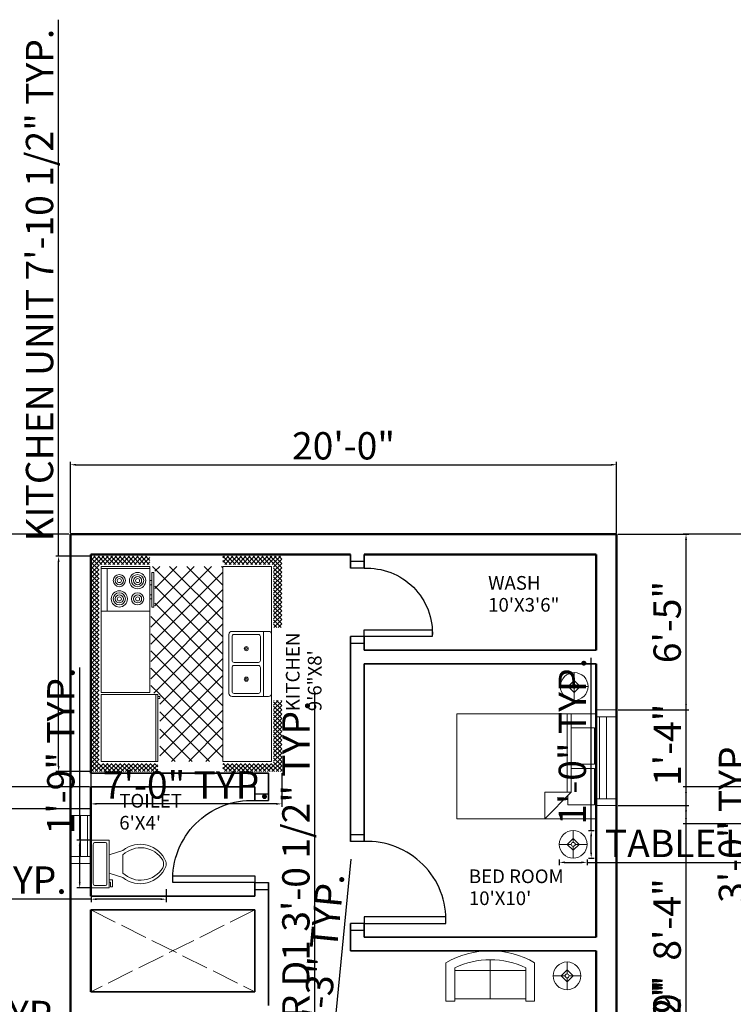
# Model space of a CAD drawing. Units: inches. Extents: x 2296 to 3335, y 495 to 1294.
# Tile 4 of 7: x 2638 to 2952, y 862 to 1294. Entities that reach past the tile are written whole.
import ezdxf

# ---------------------------------------------------------------- set-up
doc = ezdxf.new("R2010")
doc.units = ezdxf.units.IN
doc.linetypes.add('ACAD_ISO02W100', pattern=[15, 12, -3])
for name, color, linetype, lineweight in [('A-ANNO-DIMS', 2, 'Continuous', 18), ('A-AREA-IDEN', 7, 'Continuous', 18), ('A-FLOR-FIXT', 8, 'Continuous', 18), ('A-FLOR-OPEN', 7, 'ACAD_ISO02W100', 18), ('DOORS', 1, 'Continuous', 25), ('E-LITE', 2, 'Continuous', 18), ('FURNITURE', 2, 'Continuous', 18), ('INNER WALL', 6, 'Continuous', 35), ('OUTER WALL', 5, 'Continuous', 50), ('P-FIXT', 4, 'Continuous', 18), ('VENTILATOR', 4, 'Continuous', 18), ('WINDOWS', 3, 'Continuous', 18)]:
    doc.layers.add(name, color=color, linetype=linetype, lineweight=lineweight)
doc.styles.get("Standard").update_dxf_attribs({"font": 'arial.ttf'})
doc.dimstyles.new('ISO-25', dxfattribs={"dimtxt": 12, "dimasz": 2.5, "dimexe": 1.25, "dimexo": 0.625, "dimtad": 1, "dimdec": 1, "dimlunit": 3, "dimtxsty": 'Standard', "dimcen": 2.5, "dimadec": 0, "dimazin": 0, "dimtfac": 1, "dimtdec": 1, "dimtmove": 0, "dimatfit": 3, "dimfxl": 1, "dimarcsym": 0})

# ---------------------------------------------------------------- blocks, each defined once
blk = doc.blocks.new('Kitchen Layout - 7 x 8 ft')
for p, q in [((-5, 81.32), (2.68, 89)), ((-5, 83.44), (0.56, 89)), ((-5, 85.56), (-1.56, 89)), ((-5, 87.68), (-3.68, 89)), ((-1, 84.97), (-5, 88.97)), ((1.09, 85), (-2.91, 89)), ((3.21, 85), (-0.79, 89)), ((0.81, 85), (4.81, 89)), ((5.34, 85), (1.34, 89)), ((2.93, 85), (6.93, 89)), ((7.46, 85), (3.46, 89)), ((5.05, 85), (9.05, 89)), ((9.58, 85), (5.58, 89)), ((7.17, 85), (11.17, 89)), ((11.7, 85), (7.7, 89)), ((9.29, 85), (13.29, 89)), ((13.82, 85), (9.82, 89)), ((11.41, 85), (15.41, 89)), ((15.94, 85), (11.94, 89)), ((13.53, 85), (17.53, 89)), ((18.06, 85), (14.06, 89)), ((15.65, 85), (19.65, 89)), ((20.18, 85), (16.18, 89)), ((17.78, 85), (21.78, 89)), ((22.31, 85), (18.31, 89)), ((19.9, 85), (23.9, 89)), ((24.43, 85), (20.43, 89)), ((22.02, 85), (26.02, 89)), ((26.55, 85), (22.55, 89)), ((24.14, 85), (28.14, 89)), ((28.67, 85), (24.67, 89)), ((26.26, 85), (30.26, 89)), ((30.79, 85), (26.79, 89)), ((28.38, 85), (32.38, 89)), ((32.91, 85), (28.91, 89)), ((30.5, 85), (34.5, 89)), ((35.03, 85), (31.03, 89)), ((32.63, 85), (36.63, 89)), ((37.16, 85), (33.16, 89)), ((34.75, 85), (38.75, 89)), ((39.28, 85), (35.28, 89)), ((36.87, 85), (40.87, 89)), ((41.4, 85), (37.4, 89)), ((38.99, 85), (42.99, 89)), ((43.52, 85), (39.52, 89)), ((41.11, 85), (45.11, 89)), ((45.64, 85), (41.64, 89)), ((43.23, 85), (47.23, 89)), ((47.76, 85), (43.76, 89)), ((45.35, 85), (49.35, 89)), ((49.88, 85), (45.88, 89)), ((47.47, 85), (51.47, 89)), ((52, 85), (48, 89)), ((49.6, 85), (53.6, 89)), ((54.13, 85), (50.13, 89)), ((51.72, 85), (55.72, 89)), ((56.25, 85), (52.25, 89)), ((53.84, 85), (57.84, 89)), ((58.37, 85), (54.37, 89)), ((55.96, 85), (59.96, 89)), ((60.49, 85), (56.49, 89)), ((58.08, 85), (62.08, 89)), ((62.61, 85), (58.61, 89)), ((60.2, 85), (64.2, 89)), ((64.73, 85), (60.73, 89)), ((62.32, 85), (66.32, 89)), ((66.85, 85), (62.85, 89)), ((64.45, 85), (68.45, 89)), ((68.97, 85), (64.97, 89)), ((66.57, 85), (70.57, 89)), ((71.1, 85), (67.1, 89)), ((68.69, 85), (72.69, 89)), ((73.22, 85), (69.22, 89)), ((70.81, 85), (74.81, 89)), ((75.34, 85), (71.34, 89)), ((72.93, 85), (76.93, 89)), ((77.46, 85), (73.46, 89)), ((75.05, 85), (79.05, 89)), ((79.58, 85), (75.58, 89)), ((77.17, 85), (81.17, 89)), ((81.7, 85), (77.7, 89)), ((79.29, 85), (83.29, 89)), ((83.82, 85), (79.82, 89)), ((81.42, 85), (85.42, 89)), ((85.95, 85), (81.95, 89)), ((83.54, 85), (87.54, 89)), ((88.07, 85), (84.07, 89)), ((85.66, 85), (89.66, 89)), ((90.19, 85), (86.19, 89)), ((87.78, 85), (91.78, 89)), ((92.31, 85), (88.31, 89)), ((89.9, 85), (93.9, 89)), ((94.43, 85), (90.43, 89)), ((92.02, 85), (96.02, 89)), ((96.55, 85), (92.55, 89)), ((94.14, 85), (98.14, 89)), ((101, 82.67), (94.67, 89)), ((96.27, 85), (100.27, 89)), ((101, 84.79), (96.79, 89)), ((97, 83.61), (101, 87.61)), ((101, 86.92), (98.92, 89)), ((-1, 82.85), (-5, 86.85)), ((-1, 80.73), (-5, 84.73)), ((-5, 79.19), (-1, 83.19)), ((-1, 78.61), (-5, 82.61)), ((34, 84), (96, 84)), ((34, 60), (34, 84)), ((96, 84), (96, 60)), ((97, 81.49), (101, 85.49)), ((101, 80.55), (97, 84.55)), ((97, 79.37), (101, 83.37)), ((101, 78.43), (97, 82.43)), ((-5, 77.07), (-1, 81.07)), ((-1, 76.49), (-5, 80.49)), ((-5, 74.95), (-1, 78.95)), ((-1, 74.36), (-5, 78.36)), ((74, 81), (95, 81)), ((97, 77.25), (101, 81.25)), ((101, 76.31), (97, 80.31)), ((97, 75.13), (101, 79.13)), ((101, 74.19), (97, 78.19)), ((-5, 72.83), (-1, 76.83)), ((-1, 72.24), (-5, 76.24)), ((-5, 70.71), (-1, 74.71)), ((-1, 70.12), (-5, 74.12)), ((97, 73.01), (101, 77.01)), ((101, 72.07), (97, 76.07)), ((97, 70.89), (101, 74.89)), ((101, 69.95), (97, 73.95)), ((97, 68.76), (101, 72.76)), ((-5, 68.59), (-1, 72.59)), ((-1, 68), (-5, 72)), ((-5, 66.47), (-1, 70.47)), ((-1, 65.88), (-5, 69.88)), ((-5, 64.35), (-1, 68.35)), ((101, 67.82), (97, 71.82)), ((97, 66.64), (101, 70.64)), ((101, 65.7), (97, 69.7)), ((97, 64.52), (101, 68.52)), ((-1, 63.76), (-5, 67.76)), ((-5, 62.22), (-1, 66.22)), ((-1, 61.64), (-5, 65.64)), ((-5, 60.1), (-1, 64.1)), ((-1, 59.52), (-5, 63.52)), ((101, 63.58), (97, 67.58)), ((97, 62.4), (101, 66.4)), ((101, 61.46), (97, 65.46)), ((97, 60.28), (101, 64.28)), ((100.34, 60), (97, 63.34)), ((-5, 57.98), (-1, 61.98)), ((-1, 57.39), (-5, 61.39)), ((-1.73, 56), (-5, 59.27)), ((-4.86, 56), (-1, 59.86)), ((10.4, 24), (45.9, 59.5)), ((18.88, 24), (54.38, 59.5)), ((27.37, 24), (62.87, 59.5)), ((33.03, 55.11), (37.41, 59.5)), ((96, 60), (34, 60)), ((35.85, 24), (71.35, 59.5)), ((76.2, 24), (40.7, 59.5)), ((84.68, 24), (49.18, 59.5)), ((93.17, 24), (57.67, 59.5)), ((61.31, 24), (96, 58.69)), ((96, 29.65), (66.15, 59.5)), ((80, 60), (80, 59)), ((82, 59), (82, 60)), ((87, 59), (87, 60)), ((89, 60), (89, 59)), ((98.22, 60), (97, 61.22)), ((98.84, 60), (101, 62.16)), ((100.96, 60), (101, 60.04)), ((-3.85, 56), (-5, 57.15)), ((-2.74, 56), (-1, 57.74)), ((0, 57), (33, 57)), ((0, 30.57), (24.43, 55)), ((0, 39.06), (15.94, 55)), ((0, 47.54), (7.46, 55)), ((1.91, 24), (32.91, 55)), ((33.77, 24), (2.77, 55)), ((42.26, 24), (11.26, 55)), ((50.74, 24), (19.74, 55)), ((59.23, 24), (28.23, 55)), ((31, 55), (31, 56)), ((32, 55), (31, 55)), ((32, 56), (32, 55)), ((67.71, 24), (33.68, 58.04)), ((44.34, 24), (77.84, 57.5)), ((52.82, 24), (86.32, 57.5)), ((96, 38.14), (76.64, 57.5)), ((96, 46.63), (85.13, 57.5)), ((96, 55.11), (93.57, 57.54)), ((25.29, 24), (0, 49.29)), ((69.79, 24), (96, 50.21)), ((16.8, 24), (0, 40.8)), ((78.28, 24), (96, 41.72)), ((8.32, 24), (0, 32.32)), ((86.76, 24), (96, 33.24)), ((95.25, 24), (96, 24.75)), ((-5, 21.92), (-2.92, 24)), ((-5, 19.8), (-1, 23.8)), ((-1, 19.21), (-5, 23.21)), ((-5, 17.68), (-1, 21.68)), ((-1, 17.09), (-5, 21.09)), ((-5, 15.55), (-1, 19.55)), ((-1, 21.33), (-3.67, 24)), ((-1, 23.45), (-1.55, 24)), ((0, 24), (96, 24)), ((0, 0), (0, 24)), ((96, 24), (96, 0)), ((97, 22.1), (98.9, 24)), ((97, 19.97), (101, 23.97)), ((101, 19.03), (97, 23.03)), ((97, 17.85), (101, 21.85)), ((101, 16.91), (97, 20.91)), ((97, 15.73), (101, 19.73)), ((101, 21.16), (98.16, 24)), ((101, 23.28), (100.28, 24)), ((-1, 14.97), (-5, 18.97)), ((-5, 13.43), (-1, 17.43)), ((-1, 12.85), (-5, 16.85)), ((-5, 11.31), (-1, 15.31)), ((-1, 10.73), (-5, 14.73)), ((47.25, 6.5), (47.25, 18.5)), ((48.75, 18.5), (48.75, 6.5)), ((101, 14.79), (97, 18.79)), ((97, 13.61), (101, 17.61)), ((101, 12.67), (97, 16.67)), ((97, 11.49), (101, 15.49)), ((101, 10.55), (97, 14.55)), ((-5, 9.19), (-1, 13.19)), ((-1, 8.6), (-5, 12.6)), ((-5, 7.07), (-1, 11.07)), ((-1, 6.48), (-5, 10.48)), ((97, 9.37), (101, 13.37)), ((101, 8.43), (97, 12.43)), ((97, 7.25), (101, 11.25)), ((101, 6.31), (97, 10.31)), ((-5, 4.95), (-1, 8.95)), ((-1, 4.36), (-5, 8.36)), ((-5, 2.83), (-1, 6.83)), ((-1, 2.24), (-5, 6.24)), ((97, 5.12), (101, 9.12)), ((101, 4.18), (97, 8.18)), ((97, 3), (101, 7)), ((101, 2.06), (97, 6.06)), ((97, 0.88), (101, 4.88)), ((-5, 0.71), (-1, 4.71)), ((-1, 0.12), (-5, 4.12)), ((-5, -1.42), (-1, 2.58)), ((2, -5), (-5, 2)), ((-5, -3.54), (-1, 0.46)), ((96, 0), (0, 0)), ((64, 4), (32, 4)), ((93.24, -5), (101, 2.76)), ((95.36, -5), (101, 0.64)), ((101, -0.06), (97, 3.94)), ((101, -2.18), (97, 1.82)), ((-0.12, -5), (-5, -0.12)), ((-2.25, -5), (-5, -2.25)), ((-4.37, -5), (-5, -4.37)), ((-4.34, -5), (-0.34, -1)), ((-2.22, -5), (1.78, -1)), ((-0.1, -5), (3.9, -1)), ((4.12, -5), (0.12, -1)), ((2.02, -5), (6.02, -1)), ((6.24, -5), (2.24, -1)), ((4.14, -5), (8.14, -1)), ((8.36, -5), (4.36, -1)), ((6.27, -5), (10.27, -1)), ((10.48, -5), (6.48, -1)), ((8.39, -5), (12.39, -1)), ((12.6, -5), (8.6, -1)), ((10.51, -5), (14.51, -1)), ((14.73, -5), (10.73, -1)), ((12.63, -5), (16.63, -1)), ((16.85, -5), (12.85, -1)), ((14.75, -5), (18.75, -1)), ((18.97, -5), (14.97, -1)), ((16.87, -5), (20.87, -1)), ((21.09, -5), (17.09, -1)), ((18.99, -5), (22.99, -1)), ((23.21, -5), (19.21, -1)), ((21.11, -5), (25.11, -1)), ((25.33, -5), (21.33, -1)), ((23.24, -5), (27.24, -1)), ((27.45, -5), (23.45, -1)), ((25.36, -5), (29.36, -1)), ((29.57, -5), (25.57, -1)), ((27.48, -5), (30, -2.48)), ((30, -3.3), (27.7, -1)), ((29.6, -5), (30, -4.6)), ((30, -1.18), (29.82, -1)), ((66, -2.54), (67.54, -1)), ((66, -4.66), (69.66, -1)), ((69.88, -5), (66, -1.12)), ((67.76, -5), (66, -3.24)), ((67.78, -5), (71.78, -1)), ((72, -5), (68, -1)), ((69.9, -5), (73.9, -1)), ((74.12, -5), (70.12, -1)), ((72.03, -5), (76.03, -1)), ((76.24, -5), (72.24, -1)), ((74.15, -5), (78.15, -1)), ((78.36, -5), (74.36, -1)), ((76.27, -5), (80.27, -1)), ((80.49, -5), (76.49, -1)), ((78.39, -5), (82.39, -1)), ((82.61, -5), (78.61, -1)), ((80.51, -5), (84.51, -1)), ((84.73, -5), (80.73, -1)), ((82.63, -5), (86.63, -1)), ((86.85, -5), (82.85, -1)), ((84.75, -5), (88.75, -1)), ((88.97, -5), (84.97, -1)), ((86.88, -5), (90.88, -1)), ((91.09, -5), (87.09, -1)), ((89, -5), (93, -1)), ((93.21, -5), (89.21, -1)), ((91.12, -5), (95.12, -1)), ((95.34, -5), (91.34, -1)), ((97.46, -5), (93.46, -1)), ((99.58, -5), (95.58, -1)), ((101, -4.3), (97, -0.3)), ((97.48, -5), (101, -1.48)), ((99.6, -5), (101, -3.6))]:
    blk.add_line(p, q)
for points in [[(0, 56), (0, 84), (33, 84), (33, 56)], [(74, 60), (74, 84), (95, 84), (95, 60)], [(76, 58), (76, 59), (93, 59), (93, 58)]]:
    blk.add_lwpolyline(points, close=True)
for points in [[(32, 1.5), (32, 19.5)], [(33.5, 21), (62.5, 21)], [(34.5, 19.5), (46.25, 19.5)], [(49.75, 19.5), (61.5, 19.5)], [(64, 19.5), (64, 1.5)], [(33.5, 6.5), (33.5, 18.5)], [(62.5, 18.5), (62.5, 6.5)], [(46.25, 5.5), (34.5, 5.5)], [(61.5, 5.5), (49.75, 5.5)], [(62.5, 0), (33.5, 0)]]:
    blk.add_lwpolyline(points)
for centre, radius in [((80, 75), 4), ((80, 75), 3), ((89, 75), 3), ((80, 75), 2), ((80, 75), 1), ((89, 75), 2), ((89, 75), 1), ((80, 66), 3), ((80, 66), 2), ((89, 66), 4), ((89, 66), 3), ((89, 66), 2), ((80, 66), 1), ((89, 66), 1), ((40.5, 12.5), 1), ((40.5, 12.5), 0.5), ((55.5, 12.5), 1), ((55.5, 12.5), 0.5)]:
    blk.add_circle(centre, radius)
for centre, radius, start, end in [((33.5, 19.5), 1.5, 90, 180), ((34.5, 18.5), 1, 90, 180), ((46.25, 18.5), 1, 0, 90), ((49.75, 18.5), 1, 90, 180), ((61.5, 18.5), 1, 0, 90), ((62.5, 19.5), 1.5, 0, 90), ((34.5, 6.5), 1, 180, 270), ((46.25, 6.5), 1, 270, 0), ((49.75, 6.5), 1, 180, 270), ((61.5, 6.5), 1, 270, 0), ((33.5, 1.5), 1.5, 180, 270), ((62.5, 1.5), 1.5, 270, 0)]:
    blk.add_arc(centre, radius, start, end)
blk = doc.blocks.new('Toilet - top')
for p, q in [((9.5, -6), (9.5, -2)), ((-10, -8.5), (-8, -8.5)), ((-10, -9.5), (-10, -8.5)), ((-8, -8.5), (-8, -8)), ((-7, -8), (-7, -9.5)), ((-4, -8), (-6, -14)), ((4, -8), (6, -14)), ((-7, -9.5), (-10, -9.5)), ((4, -14), (-4, -14))]:
    blk.add_line(p, q)
blk.add_lwpolyline([(10.5, -8), (10.5, 0), (-10.5, 0), (-10.5, -8)], close=True)
for points in [[(-9.5, -2), (-9.5, -6)], [(8.5, -1), (-8.5, -1)], [(-8.5, -7), (8.5, -7)]]:
    blk.add_lwpolyline(points)
for centre, radius, start, end in [((-8.62, -1.88), 0.884, 81.8699, 188.1301), ((8.62, -1.88), 0.884, 351.8699, 98.1301), ((-8.62, -6.12), 0.884, 171.8699, 278.1301), ((8.62, -6.12), 0.884, 261.8699, 8.1301), ((3.52, -21.58), 12.17, 141.4691, 247.9714), ((4.2, -21.82), 11.33, 136.3677, 238.9468), ((-3.52, -21.58), 12.17, 292.0284, 38.5307), ((-4.2, -21.82), 11.33, 301.053, 43.6321), ((0, -27.88), 4, 245.7318, 294.2682), ((0, -29), 4, 254.8605, 285.1395)]:
    blk.add_arc(centre, radius, start, end)
blk = doc.blocks.new('Bed - Queen')
for p, q in [((0, -80.00003), (0, 0)), ((0, 0), (59.99999, 0)), ((59.99999, 0), (59.99999, -80.00003)), ((7.99999, -1.2), (28.79998, -1.2)), ((7.99999, -14.4), (7.99999, -1.2)), ((28.79998, -1.2), (28.79998, -14.4)), ((31.19999, -1.2), (51.99999, -1.2)), ((31.19999, -14.4), (31.19999, -1.2)), ((51.99999, -1.2), (51.99999, -16.4)), ((0, -14.4), (44.8, -14.4)), ((44.8, -16.8), (0, -16.8)), ((59.99999, -29.6), (44.8, -14.4)), ((44.8, -14.4), (44.8, -29.6)), ((51.99999, -16.4), (46.79936, -16.4)), ((44.8, -29.6), (59.99999, -29.6)), ((59.99999, -80.00003), (0, -80.00003))]:
    blk.add_line(p, q)
blk = doc.blocks.new('Lamp - Table')
for p, q in [((0, 7), (0, 1)), ((-1, 0), (-7, 0)), ((0, 3), (-3, 0)), ((-3, 0), (0, -3)), ((3, 0), (0, 3)), ((0, -3), (3, 0)), ((1, 0), (7, 0)), ((0, -1), (0, -7))]:
    blk.add_line(p, q)
for radius in [7, 1]:
    blk.add_circle((0, 0), radius)
blk = doc.blocks.new('Sofa - Roundback Loveseat 5 ft.')
for p, q in [((0, -32.44198), (0, -5.99998)), ((-24, -33.99998), (-24, -11.46958)), ((24.00004, -33.99998), (24.00004, -11.46958)), ((-23.9998, -13.38178), (23.99986, -13.38178)), ((-24, -32.44198), (24.00004, -32.44198))]:
    blk.add_line(p, q)
for points in [[(-24, -33.99998), (-30, -33.99998), (-30, -7.99998)], [(30.00004, -7.99998), (30.00004, -33.99998), (24.00004, -33.99998)]]:
    blk.add_lwpolyline(points)
for centre, radius, start, end in [((0, -60.24998), 60.24998, 60.13715, 119.8628), ((0, -61.38438), 55.38444, 64.32083, 115.6792)]:
    blk.add_arc(centre, radius, start, end)
blk = doc.blocks.new('DOOR-SINGLE-30IN')
for p, q in [((-3, 0), (-3, -6)), ((0, 0), (0, -6)), ((30, 0), (30, -6)), ((33, 0), (33, -6))]:
    blk.add_line(p, q)
blk.add_lwpolyline([(0, 0), (3, 0), (3, 30), (0, 30)], close=True)
blk.add_arc((1.5, 1.5), 28.54, 356.9872, 93.0128)
blk = doc.blocks.new('DOOR-SINGLE-36IN')
for p, q in [((0, 39), (-6, 39)), ((0, 36), (-6, 36)), ((0, 0), (-6, 0)), ((0, -3), (-6, -3))]:
    blk.add_line(p, q)
blk.add_lwpolyline([(0, 0), (36, 0), (36, 3), (0, 3)], close=True)
blk.add_arc((1.5, 1.5), 34.53, 357.5104, 92.4896)
blk = doc.blocks.new('WIN-36IN')
for p, q in [((0, 42), (9, 42)), ((0, 39), (9, 39)), ((1.5, 3), (1.5, 39)), ((4.5, 3), (4.5, 39)), ((9, 3), (0, 3)), ((9, 0), (0, 0))]:
    blk.add_line(p, q)
blk = doc.blocks.new('VENT-18IN')
for p, q in [((0, 24), (9, 24)), ((0, 21), (9, 21)), ((4.5, 21), (4.5, 3)), ((7.5, 21), (7.5, 3)), ((9, 3), (0, 3)), ((9, 0), (0, 0))]:
    blk.add_line(p, q)
blk = doc.blocks.new('FLOOR-OPENING-72X36')
for p, q in [((0, 36), (72, 0)), ((72, 36), (0, 0))]:
    blk.add_line(p, q)
blk = doc.blocks.new('*D24')
at = {"layer": 'A-ANNO-DIMS', "color": 0, "lineweight": -2, "transparency": 16777216}
for p, q in [((2959.85, 903.02), (2959.85, 979.91)), ((2970.02, 903.02), (2958.6, 903.02)), ((2959.85, 869.52), (2959.85, 900.52)), ((2970.02, 867.02), (2958.6, 867.02))]:
    blk.add_line(p, q, dxfattribs=at)
at = {"layer": 'A-ANNO-DIMS', "color": 0, "transparency": 16777216}
for points in [[(2959.43, 900.52), (2960.26, 900.52), (2959.85, 903.02)], [(2959.43, 869.52), (2960.26, 869.52), (2959.85, 867.02)]]:
    blk.add_solid(points, dxfattribs=at)
at = {"layer": 'Defpoints', "color": 0, "transparency": 16777216}
for p in [(2959.85, 903.02), (2970.65, 903.02), (2970.65, 867.02)]:
    blk.add_point(p, dxfattribs=at)
at = {"layer": 'A-ANNO-DIMS', "color": 0, "transparency": 16777216, "insert": (2953.09, 942.71), "char_height": 12, "attachment_point": 5, "rotation": 90}
blk.add_mtext('3\'-0" TYP.', dxfattribs=at)
blk = doc.blocks.new('*D25')
at = {"layer": 'A-ANNO-DIMS', "color": 0, "lineweight": -2, "transparency": 16777216}
for p, q in [((2655.47, 1058.33), (2655.47, 1293.98)), ((2669.03, 1058.33), (2654.22, 1058.33)), ((2655.47, 966.25), (2655.47, 1055.83)), ((2669.03, 963.75), (2654.22, 963.75))]:
    blk.add_line(p, q, dxfattribs=at)
at = {"layer": 'A-ANNO-DIMS', "color": 0, "transparency": 16777216}
for points in [[(2655.05, 1055.83), (2655.89, 1055.83), (2655.47, 1058.33)], [(2655.05, 966.25), (2655.89, 966.25), (2655.47, 963.75)]]:
    blk.add_solid(points, dxfattribs=at)
at = {"layer": 'Defpoints', "color": 0, "transparency": 16777216}
for p in [(2655.47, 1058.33), (2669.66, 1058.33), (2669.66, 963.75)]:
    blk.add_point(p, dxfattribs=at)
at = {"layer": 'A-ANNO-DIMS', "color": 0, "transparency": 16777216, "insert": (2648.64, 1177.41), "char_height": 12, "attachment_point": 5, "rotation": 90}
blk.add_mtext('KITCHEN UNIT 7\'-10 1/2" TYP.', dxfattribs=at)
blk = doc.blocks.new('*D26')
at = {"layer": 'A-ANNO-DIMS', "color": 0, "lineweight": -2, "transparency": 16777216}
for p, q in [((2669.66, 963.12), (2669.66, 948.31)), ((2753.53, 963.12), (2753.53, 948.31)), ((2751.03, 949.56), (2672.16, 949.56))]:
    blk.add_line(p, q, dxfattribs=at)
at = {"layer": 'A-ANNO-DIMS', "color": 0, "transparency": 16777216}
for points in [[(2672.16, 949.98), (2672.16, 949.15), (2669.66, 949.56)], [(2751.03, 949.98), (2751.03, 949.15), (2753.53, 949.56)]]:
    blk.add_solid(points, dxfattribs=at)
at = {"layer": 'Defpoints', "color": 0, "transparency": 16777216}
for p in [(2669.66, 963.75), (2753.53, 963.75), (2669.66, 949.56)]:
    blk.add_point(p, dxfattribs=at)
at = {"layer": 'A-ANNO-DIMS', "color": 0, "transparency": 16777216, "insert": (2711.59, 956.31), "char_height": 12, "attachment_point": 5}
blk.add_mtext('7\'-0" TYP.', dxfattribs=at)
blk = doc.blocks.new('*D29')
at = {"layer": 'A-ANNO-DIMS', "color": 0, "lineweight": -2, "transparency": 16777216}
for p, q in [((2875.48, 925.07), (2875.48, 922.62)), ((2877.98, 923.87), (2885.16, 923.87)), ((2887.66, 925.07), (2887.66, 922.62)), ((2887.66, 923.87), (3072.94, 923.87))]:
    blk.add_line(p, q, dxfattribs=at)
at = {"layer": 'A-ANNO-DIMS', "color": 0, "transparency": 16777216}
for points in [[(2877.98, 924.29), (2877.98, 923.45), (2875.48, 923.87)], [(2885.16, 924.29), (2885.16, 923.45), (2887.66, 923.87)]]:
    blk.add_solid(points, dxfattribs=at)
at = {"layer": 'Defpoints', "color": 0, "transparency": 16777216}
for p in [(2875.48, 925.7), (2887.66, 925.7), (2887.66, 923.87)]:
    blk.add_point(p, dxfattribs=at)
at = {"layer": 'A-ANNO-DIMS', "color": 0, "transparency": 16777216, "insert": (2981.55, 930.62), "char_height": 12, "attachment_point": 5}
blk.add_mtext('TABLE LAMP 1\'-0" TYP.', dxfattribs=at)
blk = doc.blocks.new('*D30')
at = {"layer": 'A-ANNO-DIMS', "color": 0, "lineweight": -2, "transparency": 16777216}
for p, q in [((2889.49, 937.88), (2889.49, 1013.64)), ((2888.29, 937.88), (2890.74, 937.88)), ((2889.49, 928.2), (2889.49, 935.38)), ((2888.29, 925.7), (2890.74, 925.7))]:
    blk.add_line(p, q, dxfattribs=at)
at = {"layer": 'A-ANNO-DIMS', "color": 0, "transparency": 16777216}
for points in [[(2889.08, 935.38), (2889.91, 935.38), (2889.49, 937.88)], [(2889.08, 928.2), (2889.91, 928.2), (2889.49, 925.7)]]:
    blk.add_solid(points, dxfattribs=at)
at = {"layer": 'Defpoints', "color": 0, "transparency": 16777216}
for p in [(2887.66, 937.88), (2889.49, 937.88), (2887.66, 925.7)]:
    blk.add_point(p, dxfattribs=at)
at = {"layer": 'A-ANNO-DIMS', "color": 0, "transparency": 16777216, "insert": (2882.74, 977.01), "char_height": 12, "attachment_point": 5, "rotation": 90}
blk.add_mtext('1\'-0" TYP.', dxfattribs=at)
blk = doc.blocks.new('*D31')
at = {"layer": 'A-ANNO-DIMS', "color": 0, "lineweight": -2, "transparency": 16777216}
for p, q in [((2669.71, 912.04), (2669.71, 906.46)), ((2702.75, 912.04), (2702.75, 906.46)), ((2669.71, 907.71), (2455.4, 907.71)), ((2700.25, 907.71), (2672.21, 907.71))]:
    blk.add_line(p, q, dxfattribs=at)
at = {"layer": 'A-ANNO-DIMS', "color": 0, "transparency": 16777216}
for points in [[(2672.21, 908.12), (2672.21, 907.29), (2669.71, 907.71)], [(2700.25, 908.12), (2700.25, 907.29), (2702.75, 907.71)]]:
    blk.add_solid(points, dxfattribs=at)
at = {"layer": 'Defpoints', "color": 0, "transparency": 16777216}
for p in [(2669.71, 912.66), (2702.75, 912.66), (2669.71, 907.71)]:
    blk.add_point(p, dxfattribs=at)
at = {"layer": 'A-ANNO-DIMS', "color": 0, "transparency": 16777216, "insert": (2561.3, 914.54), "char_height": 12, "attachment_point": 5}
blk.add_mtext('WATER CLOSET 2\'-9" TYP.', dxfattribs=at)
blk = doc.blocks.new('*D32')
at = {"layer": 'A-ANNO-DIMS', "color": 0, "lineweight": -2, "transparency": 16777216}
for p, q in [((2664.75, 933.66), (2664.75, 1009.43)), ((2669.08, 933.66), (2663.5, 933.66)), ((2664.75, 915.16), (2664.75, 931.16)), ((2669.08, 912.66), (2663.5, 912.66))]:
    blk.add_line(p, q, dxfattribs=at)
at = {"layer": 'A-ANNO-DIMS', "color": 0, "transparency": 16777216}
for points in [[(2664.33, 931.16), (2665.16, 931.16), (2664.75, 933.66)], [(2664.33, 915.16), (2665.16, 915.16), (2664.75, 912.66)]]:
    blk.add_solid(points, dxfattribs=at)
at = {"layer": 'Defpoints', "color": 0, "transparency": 16777216}
for p in [(2664.75, 933.66), (2669.71, 933.66), (2669.71, 912.66)]:
    blk.add_point(p, dxfattribs=at)
at = {"layer": 'A-ANNO-DIMS', "color": 0, "transparency": 16777216, "insert": (2658, 972.8), "char_height": 12, "attachment_point": 5, "rotation": 90}
blk.add_mtext('1\'-9" TYP.', dxfattribs=at)
blk = doc.blocks.new('*D37')
at = {"layer": 'A-ANNO-DIMS', "color": 0, "lineweight": -2, "transparency": 16777216}
for p, q in [((2768.12, 813.44), (2768.12, 998.74)), ((2763.28, 813.44), (2769.37, 813.44)), ((2768.12, 779.52), (2768.12, 810.94)), ((2763.28, 777.02), (2769.37, 777.02))]:
    blk.add_line(p, q, dxfattribs=at)
at = {"layer": 'A-ANNO-DIMS', "color": 0, "transparency": 16777216}
for points in [[(2767.7, 810.94), (2768.54, 810.94), (2768.12, 813.44)], [(2767.7, 779.52), (2768.54, 779.52), (2768.12, 777.02)]]:
    blk.add_solid(points, dxfattribs=at)
at = {"layer": 'Defpoints', "color": 0, "transparency": 16777216}
for p in [(2762.66, 813.44), (2768.12, 813.44), (2762.66, 777.02)]:
    blk.add_point(p, dxfattribs=at)
at = {"layer": 'A-ANNO-DIMS', "color": 0, "transparency": 16777216, "insert": (2761.28, 907.34), "char_height": 12, "attachment_point": 5, "rotation": 90}
blk.add_mtext('DOOR D1 3\'-0 1/2" TYP.', dxfattribs=at)
blk = doc.blocks.new('*D46')
at = {"layer": 'A-ANNO-DIMS', "color": 0, "lineweight": -2, "transparency": 16777216}
for p, q in [((2539.71, 845.21), (2539.71, 849.93)), ((2542.21, 848.68), (2550.88, 848.68)), ((2553.38, 845.21), (2553.38, 849.93)), ((2553.38, 848.68), (2657.11, 848.68))]:
    blk.add_line(p, q, dxfattribs=at)
at = {"layer": 'A-ANNO-DIMS', "color": 0, "transparency": 16777216}
for points in [[(2542.21, 849.1), (2542.21, 848.27), (2539.71, 848.68)], [(2550.88, 849.1), (2550.88, 848.27), (2553.38, 848.68)]]:
    blk.add_solid(points, dxfattribs=at)
at = {"layer": 'Defpoints', "color": 0, "transparency": 16777216}
for p in [(2553.38, 848.68), (2539.71, 844.58), (2553.38, 844.58)]:
    blk.add_point(p, dxfattribs=at)
at = {"layer": 'A-ANNO-DIMS', "color": 0, "transparency": 16777216, "insert": (2606.5, 855.51), "char_height": 12, "attachment_point": 5}
blk.add_mtext('1\'-1 1/2" TYP.', dxfattribs=at)
blk = doc.blocks.new('*D47')
at = {"layer": 'A-ANNO-DIMS', "color": 0, "lineweight": -2, "transparency": 16777216}
for p, q in [((2762.87, 710.27), (2784.09, 925.21)), ((2759.46, 710.6), (2764.11, 710.14)), ((2760.46, 685.88), (2762.62, 707.78)), ((2756.81, 683.73), (2761.46, 683.27))]:
    blk.add_line(p, q, dxfattribs=at)
at = {"layer": 'A-ANNO-DIMS', "color": 0, "transparency": 16777216}
for points in [[(2762.21, 707.82), (2763.04, 707.74), (2762.87, 710.27)], [(2760.04, 685.93), (2760.87, 685.84), (2760.21, 683.4)]]:
    blk.add_solid(points, dxfattribs=at)
at = {"layer": 'Defpoints', "color": 0, "transparency": 16777216}
for p in [(2758.84, 710.66), (2762.87, 710.27), (2756.18, 683.79)]:
    blk.add_point(p, dxfattribs=at)
at = {"layer": 'A-ANNO-DIMS', "color": 0, "transparency": 16777216, "insert": (2766.79, 819.65), "char_height": 12, "attachment_point": 5, "rotation": 84.3621}
blk.add_mtext('ROCKING CHAIR 2\'-3" TYP.', dxfattribs=at)
blk = doc.blocks.new('*D51')
at = {"layer": 'A-ANNO-DIMS', "color": 0, "lineweight": -2, "transparency": 16777216}
for p, q in [((2660.66, 1068.64), (2660.66, 1099.77)), ((2663.16, 1098.52), (2898.16, 1098.52)), ((2900.66, 1068.64), (2900.66, 1099.77))]:
    blk.add_line(p, q, dxfattribs=at)
at = {"layer": 'A-ANNO-DIMS', "color": 0, "transparency": 16777216}
for points in [[(2663.16, 1098.93), (2663.16, 1098.1), (2660.66, 1098.52)], [(2898.16, 1098.93), (2898.16, 1098.1), (2900.66, 1098.52)]]:
    blk.add_solid(points, dxfattribs=at)
at = {"layer": 'Defpoints', "color": 0, "transparency": 16777216}
for p in [(2900.66, 1098.52), (2660.66, 1068.02), (2900.66, 1068.02)]:
    blk.add_point(p, dxfattribs=at)
at = {"layer": 'A-ANNO-DIMS', "color": 0, "transparency": 16777216, "insert": (2780.66, 1105.27), "char_height": 12, "attachment_point": 5}
blk.add_mtext('20\'-0"', dxfattribs=at)
blk = doc.blocks.new('*D52')
at = {"layer": 'A-ANNO-DIMS', "color": 0, "lineweight": -2, "transparency": 16777216}
for p, q in [((2660.03, 1068.02), (2628.91, 1068.02)), ((2630.16, 590.52), (2630.16, 1065.52)), ((2660.03, 588.02), (2628.91, 588.02))]:
    blk.add_line(p, q, dxfattribs=at)
at = {"layer": 'A-ANNO-DIMS', "color": 0, "transparency": 16777216}
for points in [[(2629.74, 1065.52), (2630.57, 1065.52), (2630.16, 1068.02)], [(2629.74, 590.52), (2630.57, 590.52), (2630.16, 588.02)]]:
    blk.add_solid(points, dxfattribs=at)
at = {"layer": 'Defpoints', "color": 0, "transparency": 16777216}
for p in [(2630.16, 1068.02), (2660.66, 1068.02), (2660.66, 588.02)]:
    blk.add_point(p, dxfattribs=at)
at = {"layer": 'A-ANNO-DIMS', "color": 0, "transparency": 16777216, "insert": (2623.41, 828.02), "char_height": 12, "attachment_point": 5, "rotation": 90}
blk.add_mtext('40\'-0"', dxfattribs=at)
blk = doc.blocks.new('*D54')
at = {"layer": 'A-ANNO-DIMS', "color": 0, "lineweight": -2, "transparency": 16777216}
for p, q in [((2961.02, 1068.02), (2929.9, 1068.02)), ((2931.15, 590.52), (2931.15, 1065.52)), ((2961.02, 588.02), (2929.9, 588.02))]:
    blk.add_line(p, q, dxfattribs=at)
at = {"layer": 'A-ANNO-DIMS', "color": 0, "transparency": 16777216}
for points in [[(2930.73, 1065.52), (2931.56, 1065.52), (2931.15, 1068.02)], [(2930.73, 590.52), (2931.56, 590.52), (2931.15, 588.02)]]:
    blk.add_solid(points, dxfattribs=at)
at = {"layer": 'Defpoints', "color": 0, "transparency": 16777216}
for p in [(2931.15, 1068.02), (2961.65, 1068.02), (2961.65, 588.02)]:
    blk.add_point(p, dxfattribs=at)
at = {"layer": 'A-ANNO-DIMS', "color": 0, "transparency": 16777216, "insert": (2924.39, 828.02), "char_height": 12, "attachment_point": 5, "rotation": 90}
blk.add_mtext('40\'-0"', dxfattribs=at)
blk = doc.blocks.new('*D66')
at = {"layer": 'A-ANNO-DIMS', "color": 0, "lineweight": -2, "transparency": 16777216}
for p, q in [((2931.15, 837.02), (2931.15, 872.67)), ((2970.02, 837.02), (2929.9, 837.02)), ((2931.15, 830.52), (2931.15, 834.52)), ((2970.02, 828.02), (2929.9, 828.02))]:
    blk.add_line(p, q, dxfattribs=at)
at = {"layer": 'A-ANNO-DIMS', "color": 0, "transparency": 16777216}
for points in [[(2930.73, 834.52), (2931.56, 834.52), (2931.15, 837.02)], [(2930.73, 830.52), (2931.56, 830.52), (2931.15, 828.02)]]:
    blk.add_solid(points, dxfattribs=at)
at = {"layer": 'Defpoints', "color": 0, "transparency": 16777216}
for p in [(2931.15, 837.02), (2970.65, 837.02), (2970.65, 828.02)]:
    blk.add_point(p, dxfattribs=at)
at = {"layer": 'A-ANNO-DIMS', "color": 0, "transparency": 16777216, "insert": (2924.39, 856.09), "char_height": 12, "attachment_point": 5, "rotation": 90}
blk.add_mtext('0\'-9"', dxfattribs=at)
blk = doc.blocks.new('*D67')
at = {"layer": 'A-ANNO-DIMS', "color": 0, "lineweight": -2, "transparency": 16777216}
for p, q in [((2901.28, 1068.02), (2932.41, 1068.02)), ((2931.16, 993.32), (2931.16, 1065.52)), ((2901.28, 990.82), (2932.41, 990.82))]:
    blk.add_line(p, q, dxfattribs=at)
at = {"layer": 'A-ANNO-DIMS', "color": 0, "transparency": 16777216}
for points in [[(2930.74, 1065.52), (2931.57, 1065.52), (2931.16, 1068.02)], [(2930.74, 993.32), (2931.57, 993.32), (2931.16, 990.82)]]:
    blk.add_solid(points, dxfattribs=at)
at = {"layer": 'Defpoints', "color": 0, "transparency": 16777216}
for p in [(2900.66, 1068.02), (2931.16, 1068.02), (2900.66, 990.82)]:
    blk.add_point(p, dxfattribs=at)
at = {"layer": 'A-ANNO-DIMS', "color": 0, "transparency": 16777216, "insert": (2924.41, 1029.42), "char_height": 12, "attachment_point": 5, "rotation": 90}
blk.add_mtext('6\'-5"', dxfattribs=at)
blk = doc.blocks.new('*D68')
at = {"layer": 'A-ANNO-DIMS', "color": 0, "lineweight": -2, "transparency": 16777216}
for p, q in [((2901.28, 948.82), (2932.41, 948.82)), ((2931.16, 851.25), (2931.16, 946.32)), ((2901.28, 848.75), (2932.41, 848.75))]:
    blk.add_line(p, q, dxfattribs=at)
at = {"layer": 'A-ANNO-DIMS', "color": 0, "transparency": 16777216}
for points in [[(2930.74, 946.32), (2931.57, 946.32), (2931.16, 948.82)], [(2930.74, 851.25), (2931.57, 851.25), (2931.16, 848.75)]]:
    blk.add_solid(points, dxfattribs=at)
at = {"layer": 'Defpoints', "color": 0, "transparency": 16777216}
for p in [(2900.66, 948.82), (2931.16, 948.82), (2900.66, 848.75)]:
    blk.add_point(p, dxfattribs=at)
at = {"layer": 'A-ANNO-DIMS', "color": 0, "transparency": 16777216, "insert": (2924.41, 898.79), "char_height": 12, "attachment_point": 5, "rotation": 90}
blk.add_mtext('8\'-4"', dxfattribs=at)
blk = doc.blocks.new('*D69')
at = {"layer": 'A-ANNO-DIMS', "color": 0, "lineweight": -2, "transparency": 16777216}
for p, q in [((2931.16, 806.75), (2931.16, 870.85)), ((2901.28, 806.75), (2932.41, 806.75)), ((2931.16, 758.61), (2931.16, 804.25)), ((2901.28, 756.11), (2932.41, 756.11))]:
    blk.add_line(p, q, dxfattribs=at)
at = {"layer": 'A-ANNO-DIMS', "color": 0, "transparency": 16777216}
for points in [[(2930.74, 804.25), (2931.57, 804.25), (2931.16, 806.75)], [(2930.74, 758.61), (2931.57, 758.61), (2931.16, 756.11)]]:
    blk.add_solid(points, dxfattribs=at)
at = {"layer": 'Defpoints', "color": 0, "transparency": 16777216}
for p in [(2900.66, 806.75), (2931.16, 806.75), (2900.66, 756.11)]:
    blk.add_point(p, dxfattribs=at)
at = {"layer": 'A-ANNO-DIMS', "color": 0, "transparency": 16777216, "insert": (2924.33, 840.05), "char_height": 12, "attachment_point": 5, "rotation": 90}
blk.add_mtext('4\'-2 1/2"', dxfattribs=at)
blk = doc.blocks.new('*D70')
at = {"layer": 'A-ANNO-DIMS', "color": 0, "lineweight": -2, "transparency": 16777216}
for p, q in [((2630.16, 957.02), (2630.16, 1020.63)), ((2669.03, 957.02), (2628.91, 957.02)), ((2630.16, 949.9), (2630.16, 954.52)), ((2669.03, 947.4), (2628.91, 947.4))]:
    blk.add_line(p, q, dxfattribs=at)
at = {"layer": 'A-ANNO-DIMS', "color": 0, "transparency": 16777216}
for points in [[(2629.74, 954.52), (2630.57, 954.52), (2630.16, 957.02)], [(2629.74, 949.9), (2630.57, 949.9), (2630.16, 947.4)]]:
    blk.add_solid(points, dxfattribs=at)
at = {"layer": 'Defpoints', "color": 0, "transparency": 16777216}
for p in [(2630.16, 957.02), (2669.66, 957.02), (2669.66, 947.4)]:
    blk.add_point(p, dxfattribs=at)
at = {"layer": 'A-ANNO-DIMS', "color": 0, "transparency": 16777216, "insert": (2623.33, 990.07), "char_height": 12, "attachment_point": 5, "rotation": 90}
blk.add_mtext('0\'-9 1/2"', dxfattribs=at)
blk = doc.blocks.new('*D76')
at = {"layer": 'A-ANNO-DIMS', "color": 0, "lineweight": -2, "transparency": 16777216}
for p, q in [((2931.15, 957.02), (2931.15, 991.54)), ((2970.02, 957.02), (2929.9, 957.02)), ((2931.15, 943.31), (2931.15, 954.52)), ((2970.02, 940.81), (2929.9, 940.81))]:
    blk.add_line(p, q, dxfattribs=at)
at = {"layer": 'A-ANNO-DIMS', "color": 0, "transparency": 16777216}
for points in [[(2930.73, 954.52), (2931.56, 954.52), (2931.15, 957.02)], [(2930.73, 943.31), (2931.56, 943.31), (2931.15, 940.81)]]:
    blk.add_solid(points, dxfattribs=at)
at = {"layer": 'Defpoints', "color": 0, "transparency": 16777216}
for p in [(2931.15, 957.02), (2970.65, 957.02), (2970.65, 940.81)]:
    blk.add_point(p, dxfattribs=at)
at = {"layer": 'A-ANNO-DIMS', "color": 0, "transparency": 16777216, "insert": (2924.5, 975.53), "char_height": 12, "attachment_point": 5, "rotation": 90}
blk.add_mtext('1\'-4"', dxfattribs=at)

msp = doc.modelspace()

# ---------------------------------------------------------------- linework, layer by layer
at = {"layer": 'INNER WALL'}
for p, q in [((2783.66, 1059.02), (2783.66, 1053.02)), ((2783.66, 1059.02), (2783.66, 1053.02)), ((2789.66, 1059.02), (2789.66, 1053.02)), ((2783.66, 1023.02), (2783.66, 933.02)), ((2783.66, 1023.02), (2783.66, 963.02)), ((2789.66, 1023.02), (2789.66, 1017.02)), ((2891.66, 1017.02), (2789.66, 1017.02)), ((2891.66, 1011.02), (2789.66, 1011.02)), ((2789.66, 1011.02), (2789.66, 933.02)), ((2747.66, 963.02), (2669.66, 963.02)), ((2747.66, 963.02), (2747.66, 951.02)), ((2741.66, 957.02), (2669.66, 957.02)), ((2741.66, 957.02), (2741.66, 951.02)), ((2741.66, 915.02), (2741.66, 909.02)), ((2747.66, 915.02), (2747.66, 861.02)), ((2741.66, 909.02), (2669.66, 909.02)), ((2741.66, 903.02), (2669.66, 903.02)), ((2741.66, 903.02), (2741.66, 867.02)), ((2783.66, 897.02), (2783.66, 885.02)), ((2789.66, 897.02), (2789.66, 891.02)), ((2891.66, 891.02), (2789.66, 891.02)), ((2891.66, 885.02), (2783.66, 885.02)), ((2741.66, 867.02), (2669.66, 867.02))]:
    msp.add_line(p, q, dxfattribs=at)
at = {"layer": 'OUTER WALL'}
for p, q in [((2669.66, 1059.02), (2669.66, 963.02)), ((2783.66, 1059.02), (2669.66, 1059.02)), ((2891.66, 1059.02), (2789.66, 1059.02)), ((2891.66, 1017.02), (2891.66, 1059.02)), ((2891.66, 891.02), (2891.66, 1011.02)), ((2669.66, 957.02), (2669.66, 909.02)), ((2669.66, 903.02), (2669.66, 867.02)), ((2891.66, 783.02), (2891.66, 885.02))]:
    msp.add_line(p, q, dxfattribs=at)
msp.add_lwpolyline([(2765.66, 588.02), (2900.66, 588.02), (2900.66, 1068.02), (2660.66, 1068.02), (2660.66, 588.02), (2669.66, 588.02)], dxfattribs=at)

# ---------------------------------------------------------------- block references
at = {"layer": 'A-FLOR-FIXT', "xscale": 0.8922679191465929, "yscale": 0.8922679191465929, "zscale": 0.8922679191465929, "rotation": 90.00000000002456}
msp.add_blockref('Kitchen Layout - 7 x 8 ft', (2749.07, 968.21), dxfattribs=at)
at = {"layer": 'A-FLOR-OPEN'}
msp.add_blockref('FLOOR-OPENING-72X36', (2669.66, 867.02), dxfattribs=at)
at = {"layer": 'DOORS', "extrusion": (0, 0, -1), "zscale": -1, "rotation": 89.99999999999879}
msp.add_blockref('DOOR-SINGLE-30IN', (-2789.66, 1023.02), dxfattribs=at)
at = {"layer": 'DOORS', "extrusion": (0, 0, -1), "zscale": -1}
msp.add_blockref('DOOR-SINGLE-36IN', (-2741.66, 915.02), dxfattribs=at)
at = {"layer": 'DOORS'}
msp.add_blockref('DOOR-SINGLE-36IN', (2789.66, 897.02), dxfattribs=at)
at = {"layer": 'E-LITE', "xscale": 0.8700180084150424, "yscale": 0.8700180084150424, "zscale": 0.8700180084150424}
for p in [(2882.03, 1001.13), (2881.57, 931.79), (2878.89, 874.03)]:
    msp.add_blockref('Lamp - Table', p, dxfattribs=at)
at = {"layer": 'FURNITURE', "xscale": 0.7674836837443932, "yscale": 0.7674836837443932, "zscale": 0.7674836837443932, "rotation": 270}
msp.add_blockref('Bed - Queen', (2891.79, 989.09), dxfattribs=at)
at = {"layer": 'FURNITURE', "xscale": 0.6498910467683475, "yscale": 0.6498910467683475, "zscale": 0.6498910467683475}
msp.add_blockref('Sofa - Roundback Loveseat 5 ft.', (2845.14, 885.02), dxfattribs=at)
at = {"layer": 'P-FIXT', "rotation": 90}
msp.add_blockref('Toilet - top', (2669.71, 923.16), dxfattribs=at)
at = {"layer": 'VENTILATOR'}
msp.add_blockref('VENT-18IN', (2660.66, 923.4), dxfattribs=at)
at = {"layer": 'WINDOWS'}
msp.add_blockref('WIN-36IN', (2891.66, 948.82), dxfattribs=at)

# ---------------------------------------------------------------- texts
at = {"layer": 'A-AREA-IDEN'}
for s, p in [('WASH', (2844.21, 1043.63)), ('10\'X3\'6"', (2844.21, 1033.99)), ('TOILET', (2682.14, 947.92)), ("6'X4'", (2682.14, 938.28)), ('BED ROOM', (2835.75, 914.76)), ("10'X10'", (2835.75, 905.12))]:
    msp.add_text(s, height=6, dxfattribs=at).set_placement(p)
for s, p in [('KITCHEN', (2761.35, 990.28)), ('9\'6"X8\'', (2770.99, 990.28))]:
    msp.add_text(s, height=6, rotation=90, dxfattribs=at).set_placement(p)

# ---------------------------------------------------------------- dimensions: what is measured, and where the dimension line sits
at = {"layer": 'A-ANNO-DIMS'}
for base, p1, p2, angle, text, picture, middle in [((2655.47, 1058.33), (2669.66, 963.75), (2669.66, 1058.33), 90, 'KITCHEN UNIT <> TYP.', '*D25', (2648.64, 1177.41)), ((2889.49, 937.88), (2887.66, 925.7), (2887.66, 937.88), 90, '<> TYP.', '*D30', (2882.74, 977.01)), ((2664.75, 933.66), (2669.71, 912.66), (2669.71, 933.66), 90, '<> TYP.', '*D32', (2658, 972.8)), ((2768.12, 813.44), (2762.66, 777.02), (2762.66, 813.44), 90, 'DOOR D1 <> TYP.', '*D37', (2761.28, 907.34)), ((2959.85, 903.02), (2970.65, 867.02), (2970.65, 903.02), 90, '<> TYP.', '*D24', (2953.09, 942.71)), ((2669.66, 949.56), (2753.53, 963.75), (2669.66, 963.75), 180, '<> TYP.', '*D26', (2711.59, 956.31)), ((2669.71, 907.71), (2702.75, 912.66), (2669.71, 912.66), 180, 'WATER CLOSET <> TYP.', '*D31', (2561.3, 914.54)), ((2762.87, 710.27), (2756.18, 683.79), (2758.84, 710.66), 84.3621, 'ROCKING CHAIR <> TYP.', '*D47', (2766.79, 819.65))]:
    dim = msp.add_linear_dim(base=base, p1=p1, p2=p2, angle=angle, text=text, dimstyle='ISO-25', override={"dimdec": 1, "dimlfac": 1, "dimrnd": 0, "dimzin": 1, "dimdsep": 46, "dimlunit": 4, "dimfrac": 2}, dxfattribs=at)
    dim.commit()
    dim.dimension.update_dxf_attribs({"geometry": picture, "text_midpoint": middle})
dim = msp.add_linear_dim(base=(2900.66, 1098.52), p1=(2660.66, 1068.02), p2=(2900.66, 1068.02), dimstyle='ISO-25', override={"dimdec": 1, "dimlfac": 1, "dimrnd": 0, "dimzin": 1, "dimdsep": 46, "dimlunit": 4, "dimfrac": 2}, dxfattribs=at)
dim.commit()
dim.dimension.update_dxf_attribs({"geometry": '*D51', "text_midpoint": (2780.66, 1105.27)})
for base, p1, p2, picture, middle in [((2630.16, 1068.02), (2660.66, 588.02), (2660.66, 1068.02), '*D52', (2623.41, 828.02)), ((2931.16, 1068.02), (2900.66, 990.82), (2900.66, 1068.02), '*D67', (2924.41, 1029.42)), ((2931.15, 1068.02), (2961.65, 588.02), (2961.65, 1068.02), '*D54', (2924.39, 828.02)), ((2630.16, 957.02), (2669.66, 947.4), (2669.66, 957.02), '*D70', (2623.33, 990.07)), ((2931.15, 957.02), (2970.65, 940.81), (2970.65, 957.02), '*D76', (2924.5, 975.53)), ((2931.16, 948.82), (2900.66, 848.75), (2900.66, 948.82), '*D68', (2924.41, 898.79)), ((2931.15, 837.02), (2970.65, 828.02), (2970.65, 837.02), '*D66', (2924.39, 856.09)), ((2931.16, 806.75), (2900.66, 756.11), (2900.66, 806.75), '*D69', (2924.33, 840.05))]:
    dim = msp.add_linear_dim(base=base, p1=p1, p2=p2, angle=90, dimstyle='ISO-25', override={"dimdec": 1, "dimlfac": 1, "dimrnd": 0, "dimzin": 1, "dimdsep": 46, "dimlunit": 4, "dimfrac": 2}, dxfattribs=at)
    dim.commit()
    dim.dimension.update_dxf_attribs({"geometry": picture, "text_midpoint": middle})
for base, p1, p2, text, picture, middle in [((2887.66, 923.87), (2875.48, 925.7), (2887.66, 925.7), 'TABLE LAMP <> TYP.', '*D29', (2981.55, 930.62)), ((2553.38, 848.68), (2539.71, 844.58), (2553.38, 844.58), '<> TYP.', '*D46', (2606.5, 855.51))]:
    dim = msp.add_linear_dim(base=base, p1=p1, p2=p2, text=text, dimstyle='ISO-25', override={"dimdec": 1, "dimlfac": 1, "dimrnd": 0, "dimzin": 1, "dimdsep": 46, "dimlunit": 4, "dimfrac": 2}, dxfattribs=at)
    dim.commit()
    dim.dimension.update_dxf_attribs({"geometry": picture, "text_midpoint": middle})

doc.saveas('drawing.dxf')
